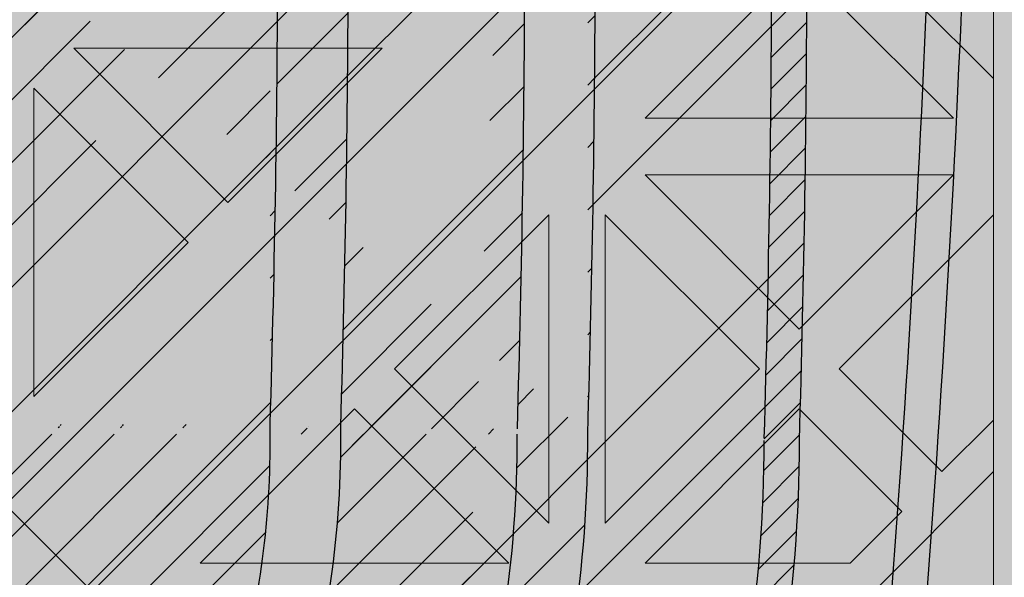
# Model space of a CAD drawing. Units: inches. Extents: x 844 to 2234, y 346 to 1084.
# Tile 54 of 93: x 1869.404 to 1873.853, y 696.327 to 698.846. Entities that reach past the tile are written whole.
import ezdxf

# ---------------------------------------------------------------- set-up
doc = ezdxf.new("R2010")
doc.units = ezdxf.units.IN
doc.header["$MEASUREMENT"] = 0
doc.layers.add('furniture', color=8, linetype='Continuous', lineweight=18)
doc.layers.add('RA-AP-01$0$INT', color=35, linetype='Continuous', lineweight=5)
doc.layers.add('RA-AP-01$0$FURN', color=3, linetype='Continuous')
doc.layers.add('RA-AP-01$0$WOOD', color=64, linetype='Continuous')

# ---------------------------------------------------------------- blocks, each defined once
blk = doc.blocks.new('A$C18D01794')
at = {"layer": 'RA-AP-01$0$INT'}
blk.add_hatch(color=256, dxfattribs=at).paths.add_polyline_path([(4.505206456958071, -6.306712009588038), (5.305206456958072, -6.306712009588038), (5.305206456958072, -7.106712009588038), (5.255206456951893, -7.10671200958804), (5.25520645694868, -6.356712009605972), (4.555206456959269, -6.356712009587461), (4.555206456956052, -7.106712009588038), (4.505206456958073, -7.106712009588038)])
h = blk.add_hatch(color=256, dxfattribs=at)
h.paths.add_polyline_path([(4.585917135068449, -6.356712009588271), (4.555206456959269, -6.35671200958746), (4.555206456959137, -6.387422687716308), (4.874495778835233, -6.706712009592356), (4.90520645695423, -6.676001331474049)])
h.paths.add_polyline_path([(5.255206456948813, -6.387422687716306), (5.255206456948682, -6.356712009605972), (5.224495778822613, -6.356712009605161), (4.905206456953498, -6.676001331474273), (4.935917135072151, -6.706712009592924)])
h.paths.add_polyline_path([(4.935917135072559, -6.706712009592068), (4.905206456953564, -6.737422687710376), (5.255206456951813, -7.087422687708613), (5.255206456951549, -7.026001331471008)])
h.paths.add_polyline_path([(4.555206456956399, -7.026001331471013), (4.555206456956134, -7.087422687708616), (4.905206456953821, -6.737422687710943), (4.874495778835166, -6.70671200959229)])
h = blk.add_hatch(color=256, dxfattribs=at)
h.paths.add_polyline_path([(4.585917135068448, -6.356712009588273), (4.614201406330596, -6.356712009589021), (4.668846067270487, -6.411356670531338), (4.723490728212344, -6.356712009591912), (4.771774999457151, -6.35671200959319), (4.826419660396886, -6.411356670535356), (4.862780050090322, -6.374996280843536), (4.844495778842715, -6.356712009595112), (4.862780050090411, -6.356712009595595), (4.905206456960182, -6.399138416468211), (4.947632863832445, -6.356712009597838), (4.965917135079675, -6.356712009598322), (4.947632863831759, -6.374996280845421), (4.983993253523576, -6.411356670538857), (5.038637914464627, -6.356712009600247), (5.08692218571208, -6.356712009601523), (5.141566846649976, -6.411356670541852), (5.196211507589851, -6.356712009604411), (5.224495778822615, -6.356712009605161), (4.905206456953975, -6.676001331473793)])
h.paths.add_polyline_path([(4.895206456956031, -6.637717060225675), (4.895206456958921, -6.528427738347902), (4.840561796018589, -6.583072399285802)], flags=16)
h.paths.add_polyline_path([(4.915206456955638, -6.637717060226121), (4.969851117895509, -6.583072399288678), (4.915206456957609, -6.528427738348344)], flags=16)
h.paths.add_polyline_path([(4.826419660395175, -6.568930263661755), (4.881064321335613, -6.514285602723745), (4.771774999456703, -6.514285602720857)], flags=16)
h.paths.add_polyline_path([(4.983993253519558, -6.568930263665262), (5.038637914460456, -6.514285602726792), (4.929348592581548, -6.514285602724816)], flags=16)
h.paths.add_polyline_path([(4.881064321336025, -6.494285602723742), (4.826419660397532, -6.439640941782821), (4.771774999457062, -6.494285602720859)], flags=16)
h.paths.add_polyline_path([(4.929348592582019, -6.494285602724817), (5.038637914460982, -6.494285602726792), (4.983993253522945, -6.439640941786327)], flags=16)
h.paths.add_polyline_path([(4.895206456960191, -6.480143467100443), (4.895206456962115, -6.407422687715913), (4.876922185715016, -6.389138416467584), (4.840561796021581, -6.425498806159401)], flags=16)
h.paths.add_polyline_path([(4.915206456958487, -6.480143467100889), (4.969851117899527, -6.425498806162279), (4.933490728206909, -6.389138416468043), (4.9152064569598, -6.40742268771434)], flags=16)
h.paths.add_polyline_path([(4.757632863832376, -6.480143467096812), (4.812277524772842, -6.425498806158772), (4.757632863834348, -6.370854145217844)], flags=16)
h.paths.add_polyline_path([(4.737632863832376, -6.480143467096286), (4.737632863834348, -6.370854145217375), (4.682988202893906, -6.425498806155385)], flags=16)
h.paths.add_polyline_path([(5.05278005008503, -6.480143467103376), (5.052780050087917, -6.370854145224413), (4.998135389146995, -6.425498806162908)], flags=16)
h.paths.add_polyline_path([(5.072780050085024, -6.480143467103744), (5.127424711025931, -6.42549880616527), (5.072780050087916, -6.370854145224832)], flags=16)
h.paths.add_polyline_path([(4.935917135072783, -6.706712009592292), (5.255206456948811, -6.387422687716309), (5.255206456948932, -6.415706958964177), (5.200561796010279, -6.470351619902839), (5.255206456949403, -6.524996280841948), (5.25520645694961, -6.5732805520894), (5.200561796009787, -6.627925213029239), (5.236922185702417, -6.664285602721864), (5.255206456949919, -6.646001331474357), (5.255206456949998, -6.664285602721898), (5.212780050078687, -6.706712009592262), (5.25520645695036, -6.749138416463932), (5.255206456950438, -6.767422687711313), (5.236922185702424, -6.749138416463297), (5.200561796009796, -6.785498806155928), (5.255206456950753, -6.840143467096874), (5.25520645695096, -6.888427738341682), (5.200561796010322, -6.943072399282328), (5.255206456951428, -6.997717060223427), (5.255206456951547, -7.026001331471006)])
h.paths.add_polyline_path([(5.042988202883395, -6.785498806155427), (5.097632863823085, -6.840143467095101), (5.097632863822622, -6.730854145216193)], flags=16)
h.paths.add_polyline_path([(5.028846067259663, -6.771356670531693), (5.083490728198774, -6.716712009592573), (4.974201406321001, -6.716712009593042)], flags=16)
h.paths.add_polyline_path([(5.117632863823087, -6.840143467095186), (5.172277524762331, -6.785498806155926), (5.11763286382262, -6.730854145216225)], flags=16)
h.paths.add_polyline_path([(5.08349072819877, -6.696712009593886), (5.028846067259652, -6.642067348654775), (4.974201406320998, -6.696712009593438)], flags=16)
h.paths.add_polyline_path([(5.131774999446817, -6.854285602718917), (5.186419660386065, -6.799640941779662), (5.241064321325782, -6.854285602719365)], flags=17)
h.paths.add_polyline_path([(5.131774999446228, -6.716712009592374), (5.186419660386065, -6.771356670532194), (5.222780050079488, -6.734996280838764), (5.204495778832781, -6.716712009592063)], flags=16)
h.paths.add_polyline_path([(5.097632863822613, -6.682569873970264), (5.097632863823061, -6.573280552091354), (5.042988202883383, -6.627925213031044)], flags=16)
h.paths.add_polyline_path([(5.131774999446899, -6.874285602718915), (5.241064321325809, -6.874285602719364), (5.186419660386591, -6.928930263658598)], flags=17)
h.paths.add_polyline_path([(5.131774999446226, -6.696712009594078), (5.204495778830767, -6.696712009594374), (5.22278005007868, -6.67842773834687), (5.186419660386049, -6.642067348654249)], flags=16)
h.paths.add_polyline_path([(5.11763286382262, -6.682569873970225), (5.17227752476232, -6.627925213030515), (5.117632863823064, -6.573280552091267)], flags=16)
h.paths.add_polyline_path([(5.186419660386069, -6.613783077405491), (5.241064321325754, -6.559138416465795), (5.131774999446791, -6.559138416466263)], flags=16)
h.paths.add_polyline_path([(5.131774999446872, -6.539138416466263), (5.24106432132578, -6.539138416465794), (5.186419660386554, -6.484493755526573)], flags=16)
h.paths.add_polyline_path([(5.255206456951811, -7.08742268770861), (5.255206456951895, -7.106712009588038), (4.555206456956052, -7.106712009588038), (4.555206456956136, -7.087422687708617), (4.905206456953973, -6.737422687710788)])
h.paths.add_polyline_path([(4.983993253513404, -6.8444937555241), (4.92934859257295, -6.899138416462108), (5.03863791445186, -6.899138416465014)], flags=16)
h.paths.add_polyline_path([(4.969851117889988, -6.83035161990006), (4.915206456952556, -6.775706958960171), (4.915206456949648, -6.884996280837944)], flags=16)
h.paths.add_polyline_path([(4.929348592572535, -6.919138416462105), (4.983993253511019, -6.973783077403037), (5.038637914451496, -6.919138416465012)], flags=16)
h.paths.add_polyline_path([(5.052780050074912, -6.93328055208906), (4.998135389134438, -6.987925213027088), (5.052780050072919, -7.042569873968025)], flags=16)
h.paths.add_polyline_path([(5.07278005007491, -6.933280552089588), (5.072780050072918, -7.042569873968497), (5.127424711013374, -6.987925213030498)], flags=16)
h.paths.add_polyline_path([(4.89520645695295, -6.775706958959721), (4.840561796013067, -6.830351619897157), (4.895206456950961, -6.884996280837494)], flags=16)
h.paths.add_polyline_path([(4.915206456948365, -6.933280552085403), (4.915206456946434, -7.006001331471951), (4.933490728192729, -7.024285602719066), (4.969851117886972, -6.987925213026453)], flags=16)
h.paths.add_polyline_path([(4.881064321327021, -6.899138416461022), (4.82641966038902, -6.84449375552057), (4.771774999448108, -6.899138416459029)], flags=16)
h.paths.add_polyline_path([(4.895206456950073, -6.933280552084951), (4.840561796009022, -6.987925213023558), (4.876922185700835, -7.024285602716997), (4.895206456948749, -7.006001331469487)], flags=16)
h.paths.add_polyline_path([(4.983993253510392, -7.0020673486505), (4.947632863816944, -7.038427738342319), (4.965917135064043, -7.05671200959023), (5.038637914448995, -7.056712009591555)], flags=16)
h.paths.add_polyline_path([(4.881064321326543, -6.91913841646102), (4.771774999447578, -6.919138416459031), (4.826419660385607, -6.973783077399508)], flags=16)
h.paths.add_polyline_path([(4.905206456946447, -7.014285602717636), (4.862780050074785, -7.056712009588352), (4.947632863816685, -7.056712009589775)], flags=16)
h.paths.add_polyline_path([(5.14156684663679, -7.002067348654549), (5.086922185696452, -7.056712009592438), (5.196211507574223, -7.056712009594425)], flags=16)
h.paths.add_polyline_path([(4.8264196603837, -7.002067348646972), (4.771774999442643, -7.056712009585575), (4.8444957788276, -7.056712009587508), (4.862780050075511, -7.038427738340416)], flags=16)
h.paths.add_polyline_path([(4.812277524760289, -6.98792521302292), (4.757632863822258, -6.933280552082447), (4.757632863819352, -7.042569873961408)], flags=16)
h.paths.add_polyline_path([(4.73763286382226, -6.933280552082079), (4.682988202881349, -6.987925213020536), (4.737632863819352, -7.04256987396099)], flags=16)
h.paths.add_polyline_path([(4.723490728195188, -7.056712009584289), (4.668846067257299, -7.002067348643949), (4.614201406317417, -7.056712009581383)], flags=16)
h.paths.add_polyline_path([(4.597632863829262, -6.706712009592262), (4.555206456957951, -6.664285602721896), (4.555206456958029, -6.646001331474357), (4.573490728205535, -6.664285602721864), (4.609851117898167, -6.627925213029238), (4.555206456958338, -6.573280552089402), (4.555206456958546, -6.524996280841952), (4.60985111789767, -6.470351619902839), (4.555206456959015, -6.415706958964177), (4.555206456959138, -6.387422687716309), (4.874495778835167, -6.70671200959229), (4.5552064569564, -7.026001331471015), (4.555206456956523, -6.997717060223433), (4.609851117897629, -6.94307239928233), (4.555206456956988, -6.888427738341681), (4.555206456957198, -6.840143467096881), (4.609851117898153, -6.78549880615593), (4.573490728205528, -6.749138416463297), (4.555206456957507, -6.76742268771132), (4.555206456957585, -6.749138416463933)])
h.paths.add_polyline_path([(4.712780050085332, -6.730854145216195), (4.712780050084863, -6.840143467095105), (4.767424711024555, -6.785498806155427)], flags=16)
h.paths.add_polyline_path([(4.726922185709173, -6.716712009592573), (4.781566846648288, -6.771356670531693), (4.836211507586949, -6.716712009593043)], flags=16)
h.paths.add_polyline_path([(4.692780050085327, -6.730854145216225), (4.638135389145619, -6.785498806155928), (4.692780050084865, -6.840143467095185)], flags=16)
h.paths.add_polyline_path([(4.726922185709182, -6.696712009593886), (4.836211507586949, -6.696712009593436), (4.7815668466483, -6.642067348654773)], flags=16)
h.paths.add_polyline_path([(4.678637914461726, -6.71671200959237), (4.605917135075169, -6.716712009592063), (4.587632863828464, -6.734996280838766), (4.623993253521887, -6.771356670532195)], flags=16)
h.paths.add_polyline_path([(4.712780050085336, -6.68256987397026), (4.767424711024568, -6.627925213031042), (4.71278005008489, -6.573280552091352)], flags=16)
h.paths.add_polyline_path([(4.678637914461726, -6.696712009594076), (4.623993253521899, -6.642067348654247), (4.587632863829271, -6.67842773834687), (4.605917135077185, -6.696712009594376)], flags=16)
h.paths.add_polyline_path([(4.692780050085336, -6.682569873970228), (4.692780050084889, -6.573280552091267), (4.638135389145632, -6.627925213030515)], flags=16)
h.paths.add_polyline_path([(4.623993253521885, -6.799640941779662), (4.678637914461131, -6.854285602718915), (4.56934859258217, -6.854285602719365)], flags=17)
h.paths.add_polyline_path([(4.623993253521901, -6.613783077405509), (4.678637914461158, -6.559138416466263), (4.569348592582195, -6.559138416465795)], flags=16)
h.paths.add_polyline_path([(4.678637914461051, -6.874285602718915), (4.623993253521361, -6.928930263658598), (4.569348592582143, -6.874285602719364)], flags=17)
h.paths.add_polyline_path([(4.678637914461076, -6.539138416466263), (4.623993253521399, -6.484493755526573), (4.569348592582167, -6.539138416465796)], flags=16)
h = blk.add_hatch(color=256, dxfattribs=at)
h.paths.add_polyline_path([(5.028846067259997, -6.642067348655121), (4.974201406321342, -6.696712009593783), (5.083490728199115, -6.69671200959423)])
h.paths.add_polyline_path([(4.974201406321344, -6.716712009593388), (5.028846067260004, -6.771356670532039), (5.083490728199117, -6.716712009592919)])
h.paths.add_polyline_path([(5.042988202883738, -6.785498806155768), (5.097632863823428, -6.840143467095449), (5.097632863822963, -6.73085414521654)])
h.paths.add_polyline_path([(5.117632863822961, -6.730854145216568), (5.117632863823428, -6.840143467095531), (5.172277524762674, -6.785498806156272)])
h.paths.add_polyline_path([(5.131774999446572, -6.716712009592718), (5.186419660386406, -6.77135667053254), (5.222780050079831, -6.734996280839116), (5.204495778833122, -6.716712009592409)])
h.paths.add_polyline_path([(5.236922185702764, -6.749138416463644), (5.200561796010139, -6.785498806156274), (5.255206456949971, -6.840143467096101), (5.255206456950271, -6.76742268771115)])
h.paths.add_polyline_path([(5.186419660386412, -6.799640941780006), (5.131774999447164, -6.854285602719262), (5.241064321326123, -6.854285602719711)])
h.paths.add_polyline_path([(5.131774999447238, -6.874285602719261), (5.186419660386934, -6.928930263658944), (5.241064321326153, -6.874285602719709)])
h.paths.add_polyline_path([(5.200561796010663, -6.943072399282675), (5.255206456949324, -6.997717060221329), (5.255206456949777, -6.888427738343558)])
h.paths.add_polyline_path([(5.21278005007903, -6.706712009592607), (5.255206456950223, -6.749138416463798), (5.255206456950696, -6.664285602721891)])
h.paths.add_polyline_path([(5.13177499944657, -6.696712009594424), (5.204495778831106, -6.696712009594723), (5.222780050079024, -6.678427738347219), (5.186419660386397, -6.642067348654592)])
h.paths.add_polyline_path([(5.117632863823405, -6.573280552091611), (5.117632863822955, -6.682569873970578), (5.172277524762665, -6.627925213030859)])
h.paths.add_polyline_path([(5.042988202883727, -6.627925213031387), (5.097632863822957, -6.682569873970603), (5.097632863823407, -6.573280552091697)])
h.paths.add_polyline_path([(5.131774999447135, -6.559138416466609), (5.186419660386394, -6.613783077405857), (5.241064321326097, -6.559138416466144)])
h.paths.add_polyline_path([(5.200561796010128, -6.627925213029584), (5.236922185702758, -6.664285602722211), (5.255206456950264, -6.646001331474705), (5.255206456949948, -6.573280552089752)])
h.paths.add_polyline_path([(5.186419660386895, -6.484493755526919), (5.131774999447213, -6.539138416466609), (5.241064321326127, -6.539138416466142)])
h.paths.add_polyline_path([(5.200561796010624, -6.470351619903183), (5.255206456949745, -6.524996280842298), (5.255206456949276, -6.415706958964523)])
h = blk.add_hatch(color=256, dxfattribs=at)
h.paths.add_polyline_path([(4.905206456953579, -6.70671200959253), (4.905206456953751, -6.676001331474523), (4.874495778835229, -6.706712009592358)])
h.paths.add_polyline_path([(4.935917135071924, -6.706712009592703), (4.905206456953583, -6.706712009592529), (4.90520645695341, -6.737422687710532)])
h = blk.add_hatch(color=256, dxfattribs=at)
h.paths.add_polyline_path([(4.895206456952951, -6.77570695895972), (4.840561796013068, -6.830351619897156), (4.895206456950958, -6.884996280837495)])
h.paths.add_polyline_path([(4.915206456949649, -6.884996280837942), (4.969851117889987, -6.830351619900054), (4.915206456952556, -6.775706958960171)])
h.paths.add_polyline_path([(5.038637914451862, -6.899138416465013), (4.983993253513403, -6.8444937555241), (4.929348592572953, -6.899138416462106)])
h.paths.add_polyline_path([(4.929348592572535, -6.919138416462105), (4.983993253511018, -6.973783077403037), (5.038637914451497, -6.919138416465012)])
h.paths.add_polyline_path([(4.915206456948366, -6.933280552085397), (4.915206456946433, -7.006001331471951), (4.93349072819273, -7.024285602719068), (4.969851117886972, -6.987925213026454)])
h.paths.add_polyline_path([(5.038637914448995, -7.056712009591553), (4.983993253510389, -7.002067348650502), (4.947632863816946, -7.038427738342318), (4.965917135064043, -7.05671200959023)])
h.paths.add_polyline_path([(5.05278005007292, -7.042569873968023), (5.05278005007491, -6.933280552089059), (4.998135389134438, -6.987925213027088)])
h.paths.add_polyline_path([(5.07278005007292, -7.042569873968496), (5.127424711013374, -6.987925213030498), (5.072780050074909, -6.933280552089588)])
h.paths.add_polyline_path([(5.141566846636789, -7.002067348654547), (5.086922185696449, -7.056712009592438), (5.196211507574223, -7.056712009594425)])
h.paths.add_polyline_path([(4.947632863816688, -7.056712009589774), (4.905206456946449, -7.014285602717634), (4.862780050074784, -7.056712009588353)])
h.paths.add_polyline_path([(4.840561796009025, -6.987925213023556), (4.876922185700834, -7.024285602716997), (4.895206456948747, -7.006001331469488), (4.895206456950075, -6.933280552084953)])
h.paths.add_polyline_path([(4.88106432132654, -6.919138416461021), (4.771774999447577, -6.919138416459031), (4.826419660385606, -6.973783077399508)])
h.paths.add_polyline_path([(4.881064321327019, -6.899138416461022), (4.826419660389019, -6.844493755520571), (4.771774999448108, -6.89913841645903)])
h.paths.add_polyline_path([(4.757632863819352, -7.042569873961409), (4.812277524760284, -6.987925213022922), (4.757632863822259, -6.933280552082447)])
h.paths.add_polyline_path([(4.8264196603837, -7.002067348646974), (4.771774999442646, -7.056712009585575), (4.844495778827599, -7.05671200958751), (4.862780050075512, -7.038427738340417)])
h.paths.add_polyline_path([(4.737632863819352, -7.042569873960988), (4.737632863822258, -6.933280552082078), (4.682988202881349, -6.987925213020538)])
h.paths.add_polyline_path([(4.668846067257299, -7.002067348643952), (4.61420140631742, -7.056712009581384), (4.723490728195189, -7.056712009584292)])
for p, q in [((5.255206456951895, -7.106712009588038), (5.255206456948681, -6.356712009605972)), ((5.25520645694988, -6.74913841646345), (5.255206456950353, -6.664285602721543)), ((4.935917135071927, -6.706712009592701), (4.905206456953407, -6.737422687710532)), ((4.935917135072783, -6.706712009592292), (5.255206456951548, -7.026001331471007)), ((5.212780050078687, -6.706712009592262), (5.25520645694988, -6.74913841646345)), ((5.083490728198772, -6.716712009592574), (4.974201406321001, -6.716712009593042)), ((4.974201406321001, -6.716712009593042), (5.028846067259663, -6.771356670531693)), ((5.08349072819877, -6.716712009592578), (5.028846067259663, -6.771356670531693)), ((5.131774999446229, -6.716712009592372), (5.186419660386063, -6.771356670532195)), ((5.204495778831181, -6.716712009592063), (5.131774999446229, -6.716712009592372)), ((5.204495778832774, -6.716712009592056), (5.222780050080282, -6.73499628083956)), ((5.09763286382262, -6.730854145216195), (5.042988202883395, -6.785498806155425)), ((5.097632863823085, -6.840143467095105), (5.09763286382262, -6.730854145216195)), ((5.11763286382262, -6.730854145216223), (5.172277524762331, -6.785498806155928)), ((5.117632863823085, -6.840143467095186), (5.11763286382262, -6.730854145216223)), ((5.186419660386062, -6.771356670532195), (5.222780050078687, -6.734996280839565)), ((4.905206456953975, -6.737422687710788), (5.255206456951811, -7.087422687708611)), ((5.200561796009796, -6.78549880615593), (5.236922185702423, -6.749138416463297)), ((5.255206456949928, -6.767422687710803), (5.236922185702423, -6.749138416463296)), ((5.236922185702423, -6.749138416463297), (5.25520645694988, -6.767422687710757)), ((5.255206456949927, -6.767422687710803), (5.255206456949628, -6.840143467095755)), ((4.915206456952556, -6.775706958960171), (4.969851117889986, -6.830351619900053)), ((4.915206456949648, -6.884996280837942), (4.915206456952556, -6.775706958960171)), ((5.042988202883397, -6.785498806155427), (5.097632863823085, -6.840143467095105)), ((5.117632863823085, -6.840143467095186), (5.172277524762331, -6.785498806155928)), ((5.255206456949628, -6.840143467095755), (5.200561796009796, -6.785498806155928)), ((5.131774999446817, -6.854285602718915), (5.186419660386065, -6.799640941779662)), ((5.24106432132578, -6.854285602719365), (5.186419660386065, -6.799640941779662)), ((4.915206456949651, -6.88499628083794), (4.969851117889986, -6.830351619900053)), ((4.929348592572952, -6.899138416462106), (4.983993253513403, -6.844493755524101)), ((4.983993253513404, -6.844493755524103), (5.038637914451862, -6.899138416465012)), ((5.131774999446817, -6.854285602718915), (5.24106432132578, -6.854285602719365)), ((5.131774999446899, -6.874285602718915), (5.241064321325809, -6.874285602719364)), ((5.186419660386587, -6.928930263658596), (5.131774999446899, -6.874285602718915)), ((5.241064321325809, -6.874285602719364), (5.186419660386589, -6.928930263658598)), ((5.255206456949429, -6.888427738343214), (5.200561796010322, -6.943072399282328)), ((5.255206456949433, -6.888427738343212), (5.255206456948982, -6.997717060220983)), ((5.038637914451862, -6.899138416465012), (4.929348592572952, -6.899138416462106))]:
    blk.add_line(p, q, dxfattribs=at)
blk = doc.blocks.new('A$C32926AE1')
at = {"layer": 'RA-AP-01$0$FURN'}
h = blk.add_hatch(dxfattribs=at)
h.set_pattern_fill('ANSI31', color=256, scale=0.1, style=0)
h.set_pattern_definition([(45, (0, 0), (-0.0088388347648318, 0.0088388347648318), [])])
edge = h.paths.add_edge_path(flags=16)
edge.add_arc((4.904771284329206, 4.246793130718756), 0.2603971832811541, 75.22398030683196, 104.7760196931204)
edge.add_arc((4.904771284329206, 4.246793130718756), 0.2603971832811541, 75.223980306832, 104.77601969312039, ccw=False)
edge = h.paths.add_edge_path(flags=16)
edge.add_arc((4.904771284329206, 4.067062675376612), 0.2603971832811541, 255.2239803068796, 284.776019693168)
edge.add_arc((4.904771284329206, 4.067062675376612), 0.2603971832811541, 255.22398030687958, 284.77601969316805, ccw=False)
edge = h.paths.add_edge_path(flags=0)
edge.add_arc((4.904771284329206, 4.067062675376612), 0.2603971832811541, 255.2239803068796, 284.776019693168)
edge.add_arc((4.904771284329206, 4.067062675376612), 0.2603971832811541, 255.22398030687958, 284.77601969316805, ccw=False)
edge = h.paths.add_edge_path(flags=0)
edge.add_arc((4.904771284329206, 4.067062675376612), 0.2603971832811541, 255.2239803068796, 284.776019693168)
edge.add_arc((4.904771284329206, 4.067062675376612), 0.2603971832811541, 255.22398030687958, 284.77601969316805, ccw=False)
edge = h.paths.add_edge_path()
edge.add_arc((4.604388392048174, 4.588829985554312), 0.1599999999999918, 342.3781640246255, 354.4317409793762)
edge.add_arc((5.090145208887507, 4.43216705527679), 0.3503971832811637, 162.0091218307731, 180.3186872093483)
edge.add_arc((5.205154176610243, 4.588829985554953), 0.1599999999999917, 185.5682590208461, 197.6218359767349)
edge.add_arc((4.904771284329229, 4.246793130718735), 0.3503971832811761, 72.00912183053516, 107.9908781690354)
edge.add_arc((9.535952835716557, 4.28682295566602), 4.798342501046485, 178.2875002453811, 181.5576802719453)
edge.add_arc((4.719397359771122, 4.43216705527679), 0.3503971832811637, 359.6813127906516, 377.9908781692269)
edge.add_arc((9.535967292294904, 4.286822350292874), 4.778371420254705, 178.2965938931842, 181.5667745797229)
edge.add_arc((4.719397359771122, 4.43216705527679), 0.3303971832811637, 359.6813127906516, 377.9908781692269)
edge.add_arc((0.2735752763637294, 4.286822350292874), 4.7783714202547, 358.4332254202771, 361.7034061068158)
edge.add_arc((5.061434214606998, 4.732549947558029), 0.1600000000000254, 252.3781640250584, 264.4317409792362)
edge.add_arc((4.748108354051257, 4.732549947558012), 0.1600000000000541, 275.5682590208426, 287.6218359759532)
edge.add_arc((4.604388392048115, 4.588829985554317), 0.1800000000000505, 342.3567572500182, 349.3735009646207)
edge.add_arc((5.205154176610254, 4.588829985554976), 0.1800000000000069, 190.6264990356027, 197.6432427513933)
edge.add_arc((5.061434214607106, 4.732549947558013), 0.1800000000000424, 252.3567572496606, 259.3735009644582)
edge.add_arc((4.904771284329208, 4.246793130718737), 0.3303971832811676, 71.99844483668534, 108.0015551637021)
edge.add_arc((4.748108354051414, 4.732549947558045), 0.1800000000000547, 280.6264990355479, 287.6432427495938)
edge.add_arc((5.090145208887514, 4.432167055276789), 0.2803971832811691, 162.8706300666893, 180.816523289902)
edge.add_arc((4.719397359771136, 4.432167055276689), 0.2803971832811534, 359.183476710103, 377.1293699333214)
edge.add_arc((4.904771284329222, 4.246793130718737), 0.2803971832811769, 72.87063006672916, 107.1293699332334)
edge.add_arc((5.090145208887522, 4.432167055276788), 0.2603971832811776, 165.2239803068007, 180.9953123810312)
edge.add_arc((4.719397359771141, 4.432167055276699), 0.2603971832811458, 359.0046876189768, 374.7760196932087)
edge.add_arc((5.090145208887507, 4.43216705527679), 0.3303971832811637, 162.0091218307731, 180.3186872093483)
edge.add_arc((9.53595427642584, 4.285015535491528), 4.728345371032053, 178.265043920078, 181.5679956281801)
edge.add_arc((0.2735882922327999, 4.285015535491582), 4.728345371032045, 358.4320043718193, 361.7349560799204)
edge.add_arc((9.535953591267507, 4.284458026472751), 4.708343996644348, 178.2573054306777, 181.5704995759608)
edge.add_arc((0.273588977391114, 4.284458026472785), 4.708343996644358, 358.4295004240388, 361.7426945693213)
edge.add_arc((0.2735889773911131, 4.029397779622582), 4.708343996644359, 358.2573054306787, 361.5704995759613)
edge.add_arc((9.535953591267518, 4.029397779622618), 4.708343996644359, 178.4295004240391, 181.7426945693223)
edge.add_arc((0.2735882922327901, 4.028840270603786), 4.728345371032054, 358.2650439200796, 361.5679956281808)
edge.add_arc((9.53595427642584, 4.028840270603841), 4.728345371032054, 178.4320043718199, 181.7349560799219)
edge.add_arc((0.2735752763637302, 4.027033455802493), 4.778371420254699, 358.2965938931842, 361.5667745797229)
edge.add_arc((4.719397359771122, 3.881688750818578), 0.3303971832811637, 342.0091218307731, 360.3186872093484)
edge.add_arc((5.090145208887507, 3.881688750818578), 0.3303971832811637, 179.6813127906516, 197.9908781692269)
edge.add_arc((9.535967292294904, 4.027033455802493), 4.778371420254705, 178.433225420277, 181.7034061068158)
edge.add_arc((4.719397359771122, 3.881688750818578), 0.3503971832811637, 342.0091218307731, 360.3186872093484)
edge.add_arc((9.53595283571655, 4.027032850429349), 4.79834250104648, 178.4423197280546, 181.7124997546188)
edge.add_arc((4.719397359771141, 3.881688750818669), 0.2603971832811458, 345.2239803067913, 360.9953123810232)
edge.add_arc((5.090145208887522, 3.88168875081858), 0.2603971832811776, 179.0046876189687, 194.7760196931993)
edge.add_arc((4.904771284329222, 4.067062675376631), 0.2803971832811769, 252.8706300667665, 287.1293699332708)
edge.add_arc((4.719397359771136, 3.881688750818678), 0.2803971832811534, 342.8706300666787, 360.8165232898969)
edge.add_arc((5.090145208887514, 3.881688750818579), 0.2803971832811691, 179.183476710098, 197.1293699333106)
edge.add_arc((4.748108354051414, 3.581305858537323), 0.1800000000000547, 72.3567572504062, 79.37350096445199)
edge.add_arc((4.904771284329208, 4.067062675376631), 0.3303971832811676, 251.9984448362979, 288.0015551633146)
edge.add_arc((5.061434214607106, 3.581305858537355), 0.1800000000000424, 100.6264990355418, 107.6432427503394)
edge.add_arc((5.205154176610254, 3.725025820540392), 0.1800000000000069, 162.3567572486066, 169.3735009643972)
edge.add_arc((4.604388392048115, 3.725025820541051), 0.1800000000000505, 10.62649903537925, 17.64324274998182)
edge.add_arc((4.748108354051257, 3.581305858537356), 0.1600000000000541, 72.37816402404681, 84.43174097915735)
edge.add_arc((4.904771284329229, 4.067062675376632), 0.3503971832811761, 252.0091218309645, 287.9908781694648)
edge.add_arc((5.061434214606998, 3.581305858537339), 0.1600000000000254, 95.56825902076373, 107.6218359749416)
edge.add_arc((5.205154176610243, 3.725025820540414), 0.1599999999999917, 162.3781640232651, 174.4317409791539)
edge.add_arc((5.090145208887507, 3.881688750818578), 0.3503971832811637, 179.6813127906516, 197.9908781692269)
edge.add_arc((4.604388392048174, 3.725025820541056), 0.1599999999999918, 5.568259020623824, 17.62183597537444)
edge.add_arc((0.2735897329420762, 4.28682295566602), 4.798342501046482, 358.4423197280547, 361.7124997546188)
edge.add_arc((0.2735897329420691, 4.027032850429348), 4.798342501046489, 358.2875002453812, 361.5576802719453)
at = {"layer": 'RA-AP-01$0$WOOD'}
h = blk.add_hatch(color=256, dxfattribs=at)
h.dxf.hatch_style = 1
h.paths.add_polyline_path([(5.157430609644524, 4.573483066760929, -0.1009492694046607), (5.155401577623758, 4.593365984175333, -0.1842662638101597), (5.172249623284174, 4.638795604568598, 0.2056608120311276), (5.179560981299304, 4.661316324430096, 0.3614336704623542), (5.134352340494423, 4.706524965234944, 0.2056608120311297), (5.111831620632933, 4.699213607219793, -0.1842662638101113), (5.066402000239693, 4.682365561559342, -0.1055311479399994), (5.045656153913092, 4.68467289944697, 0.1567636581983829), (4.763886414745334, 4.684672899446966, -0.1055311479399895), (4.743140568418733, 4.68236556155934, -0.1842662638100833), (4.6977109480255, 4.69921360721979, 0.2056608120302612), (4.675190228164109, 4.706524965234949, 0.3614336704708441), (4.629981587358889, 4.66131632442871, 0.2056608120245944), (4.637292945374126, 4.638795604567974, -0.1842662638101024), (4.654140991034615, 4.59336598417475, -0.1009492694055169), (4.652111959013835, 4.573483066760181, 0.021410119221476), (4.629748025606143, 4.156712009541676, 0.0214101192214795), (4.652111959013809, 3.739940952323101, -0.1009492694059586), (4.654140991034615, 3.720058034908448, -0.1842662638100975), (4.637292945374126, 3.674628414515226, 0.2056608120245705), (4.629981587358889, 3.652107694654492, 0.3614336704708879), (4.675190228164113, 3.606899053848249, 0.2056608120302384), (4.697710948025501, 3.614210411863408, -0.1842662638100995), (4.743140568418738, 3.63105845752386, -0.1055311479402541), (4.763886414745388, 3.628751119636215, 0.1567636581983776), (5.045656153913137, 3.628751119636244, -0.1055311479397538), (5.066402000239692, 3.631058457523857, -0.1842662638101067), (5.111831620632931, 3.614210411863407, 0.2056608120310924), (5.134352340494417, 3.606899053848256, 0.3614336704624001), (5.179560981299307, 3.652107694653103, 0.2056608120311314), (5.172249623284175, 3.6746284145146, -0.1842662638101402), (5.155401577623758, 3.72005803490786, -0.1009492694051366), (5.15743060964455, 3.739940952322354, 0.0214101192215073), (5.179794543052287, 4.156712009541468, 0.0214101192215252)])
h.paths.add_polyline_path([(4.639748609479751, 4.156712009541513, 0.0213537860821624), (4.661970494867118, 3.741887061152232, -0.094075836301374), (4.664143710413708, 3.7196126951003, -0.1824818158568985), (4.644813765429836, 3.668037719127816, 0.2056608120245319), (4.639939526753007, 3.653023905887301, 0.3614336704710246), (4.676106439397173, 3.616856993242342, 0.2056608120302234), (4.691120252638095, 3.621731231919122, -0.1824818158602558), (4.742695228611606, 3.641061176902986, -0.1029891339458722), (4.766991894714349, 3.638256818950944, 0.156709409989566), (5.042550673941472, 3.638256818950105, -0.102989133958497), (5.066847340047078, 3.641061176902949, -0.1824818158594995), (5.118422316020358, 3.621731231919103, 0.2056608120311416), (5.133436129261316, 3.616856993242346, 0.3614336704621468), (5.169603041905217, 3.653023905886178, 0.2056608120310986), (5.164728803228477, 3.668037719127177, -0.1824818158565612), (5.145398858244737, 3.719612695099578, -0.0940758363009313), (5.147572073791232, 3.741887061151398, 0.0213537860822023), (5.169793959178681, 4.156712009541451, 0.0213537860822226), (5.147572073791203, 4.571536957931898, -0.0940758363005034), (5.145398858244737, 4.59381132398362, -0.1824818158565587), (5.164728803228476, 4.645386299956021, 0.2056608120311045), (5.169603041905216, 4.66040011319702, 0.3614336704621845), (5.133436129261313, 4.696567025840856, 0.2056608120310773), (5.118422316020359, 4.691692787164098, -0.182481815859508), (5.066847340047078, 4.67236284218025, -0.1029891339584606), (5.04255067394148, 4.675167200133092, 0.156709409989566), (4.766991894714357, 4.675167200132257, -0.1029891339458842), (4.742695228611611, 4.672362842180213, -0.1824818158602725), (4.691120252638095, 4.691692787164077, 0.2056608120302152), (4.676106439397174, 4.696567025840858, 0.3614336704710363), (4.639939526753005, 4.660400113195899, 0.2056608120245495), (4.644813765429837, 4.645386299955384, -0.1824818158568934), (4.664143710413708, 4.593811323982902, -0.0940758363009187), (4.661970494867149, 4.571536957931074, 0.021353786082177)], flags=16)
h.paths.add_polyline_path([(5.129794543052235, 4.432167055276933, -0.0141661062790638), (5.130152669293814, 4.156927903047693, -0.0141661062790647), (5.129794543052234, 3.881688750818433, -0.0785247771143638), (5.10979738006795, 3.755143611847103, 0.0945969212073497), (5.105408519571111, 3.717898134952927, 0.1043170707844957), (5.116074640131521, 3.670385395016088, 0.1043170707864965), (5.068561900193738, 3.681051515576561, 0.09459692119553), (5.031316423304057, 3.676662655080835, -0.1580239521427272), (4.778226145355827, 3.676662655080367, 0.0945969211986668), (4.740980668464973, 3.681051515576592, 0.1043170707882822), (4.693467928526415, 3.670385395015844, 0.1043170707867916), (4.704134049087309, 3.717898134953662, 0.0945969211972894), (4.69974518859162, 3.755143611844042, -0.0785247771163196), (4.679748025606343, 3.881688750818406, -0.0141661062790663), (4.679389899364763, 4.156927903047693, -0.0141661062790672), (4.679748025606343, 4.432167055276998, -0.0785247771163064), (4.699745188591625, 4.55871219425134, 0.094596921197333), (4.704134049087308, 4.595957671141738, 0.1043170707867205), (4.693467928526416, 4.643470411079523, 0.1043170707882628), (4.740980668464965, 4.632804290518776, 0.0945969211988114), (4.778226145355874, 4.637193151015016, -0.158023952142669), (5.031316423304015, 4.637193151014546, 0.0945969211956361), (5.068561900193736, 4.632804290518806, 0.1043170707864979), (5.11607464013152, 4.643470411079278, 0.1043170707844617), (5.105408519571112, 4.595957671142455, 0.0945969212074597), (5.109797380067959, 4.558712194248236, -0.0785247771143467)], flags=0)
h.paths.add_polyline_path([(5.119794532311105, 4.432259799204851, -0.0142000800617244), (5.120156169157484, 4.156927903047701, -0.0142000800617277), (5.119794532311105, 3.881596006890482, -0.0784894509520253), (5.100273383573699, 3.758192358677797, 0.0940138827242913), (5.095413455884425, 3.717477693979438, 0.0606271852308753), (5.099615656341024, 3.686844378806616, 0.0606271852322524), (5.068982341167493, 3.691046579263239, 0.0940138827010453), (5.028267676478798, 3.686186651576848, -0.1580706864508061), (4.781274892180912, 3.686186651576435, 0.0940138827026903), (4.740560227491556, 3.691046579263279, 0.0606271852339895), (4.709926912317155, 3.686844378806508, 0.0606271852329405), (4.714129112773991, 3.717477693980356, 0.094013882701304), (4.709269185087677, 3.758192358669163, -0.0784894509577193), (4.689748036347473, 3.881596006890469, -0.014200080061729), (4.689386399501094, 4.156927903047709, -0.0142000800617217), (4.689748036347473, 4.432259799204808, -0.078489450957724), (4.709269185087651, 4.555663447426125, 0.0940138827014585), (4.714129112773992, 4.596378112114996, 0.0606271852329731), (4.709926912317154, 4.62701142728886, 0.0606271852340196), (4.74056022749157, 4.622809226832087, 0.0940138827024997), (4.781274892180847, 4.627669154518912, -0.1580706864508359), (5.028267676478777, 4.627669154518526, 0.0940138827010946), (5.068982341167492, 4.622809226832129, 0.060627185232254), (5.099615656341024, 4.627011427288751, 0.0606271852308727), (5.095413455884425, 4.59637811211593, 0.0940138827241088), (5.100273383573675, 4.555663447417647, -0.0784894509520978)], flags=0)
h.paths.add_polyline_path([(5.06978912287499, 4.430218106756144, -0.014241683694547), (5.070173729147532, 4.156927903047672, -0.0142416836945458), (5.06978912287499, 3.883637699339223, -0.0800609523125196), (5.052662118612511, 3.773463122773442, 0.0526421978001116), (5.04590916754064, 3.740550867606997, 0.0526421977992423), (5.012996912374707, 3.73379791653534, -0.1583028414718258), (4.796545656286308, 3.73379791653451, 0.0526421978034211), (4.763633401117837, 3.740550867607021, 0.0526421978018622), (4.756880450045755, 3.773463122774558, -0.0800609523117106), (4.739753445783639, 3.883637699339268, -0.0142416836945435), (4.739368839511098, 4.156927903047671, -0.0142416836945477), (4.739753445783639, 4.430218106756155, -0.0800609523116345), (4.75688045004574, 4.540392683320762, 0.052642197801941), (4.763633401117837, 4.573304938488346, 0.0526421978035071), (4.796545656286361, 4.580057889560873, -0.1583028414717561), (5.012996912374669, 4.580057889560039, 0.0526421977993048), (5.04590916754064, 4.57330493848837, 0.0526421978002057), (5.052662118612529, 4.540392683321868, -0.080060952312477)], flags=0)
h.paths.add_polyline_path([(5.049789715110557, 4.43038092723357, -0.0143097550741839), (5.05018085590259, 4.156927903047715, -0.0143097550741854), (5.049789715110558, 3.883474878861827, -0.0800685599149176), (5.03362098255317, 3.779581877367999, 0.0306258898956367), (5.028241146483733, 3.758218888663947, 0.0306258898977031), (5.006878157778253, 3.75283905259408, -0.1583983521624096), (4.802664410878162, 3.752839052594731, 0.0306258898946014), (4.781301422174808, 3.758218888663924, 0.0306258898967912), (4.775921586105202, 3.779581877368794, -0.080068559914251), (4.759752853548071, 3.883474878861786, -0.0143097550741854), (4.759361712756037, 4.156927903047671, -0.0143097550741854), (4.759752853548071, 4.430380927233557, -0.0800685599142479), (4.775921586105193, 4.534273928726546, 0.0306258898968306), (4.781301422174808, 4.555636917431444, 0.0306258898945754), (4.802664410878143, 4.561016753500631, -0.1583983521624168), (5.006878157778244, 4.561016753501291, 0.0306258898977177), (5.028241146483733, 4.555636917431421, 0.0306258898958182), (5.03362098255321, 4.534273928727244, -0.080068559914796)], flags=0)
h.paths.add_polyline_path([(4.999766070382627, 4.428171244713864, -0.0143443147609634), (5.000198441819402, 4.156927903047689, -0.0143443147609612), (4.999766070382627, 3.885684561381556, -0.0784641635803329), (4.987356730658798, 3.799103304488872, -0.1506053783831347), (4.822185837999821, 3.79910330448882, -0.0784641635803318), (4.809776498276007, 3.885684561381509, -0.014344314760963), (4.809344126839227, 4.156927903047677, -0.0143443147609645), (4.809776498276007, 4.428171244713873, -0.0784641635803192), (4.822185837999822, 4.514752501606549, -0.1506053783831338), (4.987356730658798, 4.514752501606494, -0.078464163580285)], flags=0)
h.paths.add_polyline_path([(4.979755254238824, 4.42764379880488, -0.0143772539198268), (4.980205517789977, 4.156927903047693, -0.0143772539198275), (4.979755254238824, 3.886212007290489, -0.0689242507424422), (4.971183264704897, 3.815276770442801, -0.1296645318904179), (4.838359303953726, 3.815276770442746, -0.0689242507424186), (4.829787314419809, 3.886212007290419, -0.0143772539198292), (4.829337050868653, 4.156927903047653, -0.0143772539198325), (4.829787314419809, 4.427643798804946, -0.0689242507424211), (4.838359303953725, 4.498579035652621, -0.1296645318904187), (4.971183264704897, 4.498579035652565, -0.0689242507424401)], flags=0)
h = blk.add_hatch(color=256, dxfattribs=at)
h.dxf.hatch_style = 1
h.paths.add_polyline_path([(5.145398858244737, 4.59381132398362, -0.1824818158565616), (5.164728803228476, 4.645386299956021, 0.2056608120311045), (5.169603041905216, 4.66040011319702, 0.3614336704621845), (5.133436129261313, 4.696567025840856, 0.2056608120310773), (5.118422316020359, 4.691692787164098, -0.182481815859508), (5.066847340047078, 4.67236284218025, -0.1029891339584606), (5.04255067394148, 4.675167200133092, 0.156709409989566), (4.766991894714357, 4.675167200132257, -0.1029891339458842), (4.742695228611611, 4.672362842180213, -0.1824818158602725), (4.691120252638095, 4.691692787164077, 0.2056608120302152), (4.676106439397174, 4.696567025840858, 0.3614336704710363), (4.639939526753005, 4.660400113195899, 0.2056608120245495), (4.644813765429837, 4.645386299955384, -0.1824818158568934), (4.664143710413708, 4.593811323982902, -0.0940758363009187), (4.661970494867149, 4.571536957931074, 0.0213537860821772), (4.639748609479751, 4.156712009541507, 0.0213537860821625), (4.661970494867119, 3.741887061152226, -0.0940758363013071), (4.664143710413708, 3.719612695100309, -0.1824818158569294), (4.644813765429836, 3.668037719127816, 0.2056608120245319), (4.639939526753007, 3.653023905887301, 0.3614336704710246), (4.676106439397173, 3.616856993242342, 0.2056608120302234), (4.691120252638095, 3.621731231919122, -0.1824818158602558), (4.742695228611606, 3.641061176902986, -0.1029891339458722), (4.766991894714349, 3.638256818950944, 0.156709409989566), (5.042550673941472, 3.638256818950105, -0.102989133958497), (5.066847340047078, 3.641061176902949, -0.1824818158594995), (5.118422316020358, 3.621731231919103, 0.2056608120311416), (5.133436129261316, 3.616856993242346, 0.3614336704621468), (5.169603041905217, 3.653023905886178, 0.2056608120310986), (5.164728803228477, 3.668037719127177, -0.1824818158565612), (5.145398858244737, 3.719612695099578, -0.0940758363009313), (5.147572073791232, 3.741887061151398, 0.0213537860822023), (5.169793959178681, 4.156712009541451, 0.0213537860822226), (5.147572073791203, 4.571536957931898, -0.0940758363004996)])
h.paths.add_polyline_path([(5.109797380067958, 4.55871219424824, -0.0785247771143472), (5.129794543052234, 4.432167055276936, -0.0141661062790644), (5.130152669293814, 4.156927903047685, -0.014166106279066), (5.129794543052234, 3.881688750818401, -0.0785247771143517), (5.109797380067946, 3.755143611847092, 0.0945969212073132), (5.105408519571111, 3.717898134952929, 0.1043170707844995), (5.116074640131521, 3.670385395016088, 0.1043170707864965), (5.068561900193738, 3.681051515576561, 0.09459692119553), (5.031316423304057, 3.676662655080835, -0.1580239521427272), (4.778226145355827, 3.676662655080367, 0.0945969211986668), (4.740980668464973, 3.681051515576592, 0.1043170707882822), (4.693467928526415, 3.670385395015844, 0.1043170707867916), (4.704134049087309, 3.717898134953662, 0.0945969211972894), (4.69974518859162, 3.755143611844042, -0.0785247771163196), (4.679748025606343, 3.881688750818406, -0.0141661062790663), (4.679389899364763, 4.156927903047693, -0.0141661062790672), (4.679748025606343, 4.432167055276998, -0.0785247771163064), (4.699745188591625, 4.55871219425134, 0.094596921197333), (4.704134049087308, 4.595957671141738, 0.1043170707867205), (4.693467928526416, 4.643470411079523, 0.1043170707882628), (4.740980668464965, 4.632804290518776, 0.0945969211988114), (4.778226145355874, 4.637193151015016, -0.158023952142669), (5.031316423304015, 4.637193151014546, 0.0945969211956361), (5.068561900193736, 4.632804290518806, 0.1043170707864979), (5.11607464013152, 4.643470411079278, 0.1043170707844617), (5.105408519571112, 4.595957671142455, 0.0945969212074504)], flags=16)
h.paths.add_polyline_path([(5.100273383573655, 4.55566344741771, -0.0784894509521388), (5.119794532311105, 4.432259799204852, -0.0142000800617252), (5.120156169157484, 4.156927903047686, -0.014200080061726), (5.119794532311105, 3.881596006890502, -0.0784894509520446), (5.100273383573696, 3.758192358677786, 0.0940138827242721), (5.095413455884425, 3.717477693979436, 0.0606271852308692), (5.099615656341024, 3.686844378806616, 0.0606271852322522), (5.068982341167493, 3.691046579263239, 0.0940138827010453), (5.028267676478798, 3.686186651576848, -0.1580706864508061), (4.781274892180912, 3.686186651576435, 0.0940138827026903), (4.740560227491556, 3.691046579263279, 0.0606271852339895), (4.709926912317155, 3.686844378806508, 0.0606271852329405), (4.714129112773991, 3.717477693980356, 0.094013882701304), (4.709269185087677, 3.758192358669163, -0.0784894509577193), (4.689748036347473, 3.881596006890469, -0.014200080061729), (4.689386399501094, 4.156927903047709, -0.0142000800617217), (4.689748036347473, 4.432259799204808, -0.078489450957724), (4.709269185087651, 4.555663447426125, 0.0940138827014585), (4.714129112773992, 4.596378112114996, 0.0606271852329731), (4.709926912317154, 4.62701142728886, 0.0606271852340196), (4.74056022749157, 4.622809226832087, 0.0940138827024997), (4.781274892180847, 4.627669154518912, -0.1580706864508359), (5.028267676478777, 4.627669154518526, 0.0940138827010946), (5.068982341167492, 4.622809226832129, 0.060627185232254), (5.099615656341024, 4.627011427288751, 0.0606271852308727), (5.095413455884425, 4.59637811211593, 0.094013882723957)], flags=0)
h.paths.add_polyline_path([(5.04590916754064, 4.57330493848837, 0.0526421978002057), (5.052662118612529, 4.540392683321868, -0.0800609523124783), (5.06978912287499, 4.430218106756142, -0.0142416836945469), (5.070173729147532, 4.156927903047672, -0.0142416836945458), (5.06978912287499, 3.883637699339223, -0.0800609523125196), (5.052662118612511, 3.773463122773442, 0.0526421978001116), (5.04590916754064, 3.740550867606997, 0.0526421977992423), (5.012996912374707, 3.73379791653534, -0.1583028414718258), (4.796545656286308, 3.73379791653451, 0.0526421978034211), (4.763633401117837, 3.740550867607021, 0.0526421978018622), (4.756880450045755, 3.773463122774558, -0.0800609523117106), (4.739753445783639, 3.883637699339268, -0.0142416836945435), (4.739368839511098, 4.156927903047671, -0.0142416836945477), (4.739753445783639, 4.430218106756155, -0.0800609523116345), (4.75688045004574, 4.540392683320762, 0.052642197801941), (4.763633401117837, 4.573304938488346, 0.0526421978035071), (4.796545656286361, 4.580057889560873, -0.1583028414717561), (5.012996912374669, 4.580057889560039, 0.0526421977993048)], flags=0)
h.paths.add_polyline_path([(5.028241146483733, 4.555636917431422, 0.0306258898956949), (5.033620982553182, 4.534273928727329, -0.0800685599148649), (5.049789715110557, 4.430380927233569, -0.0143097550741839), (5.05018085590259, 4.156927903047715, -0.0143097550741854), (5.049789715110558, 3.883474878861827, -0.0800685599149176), (5.03362098255317, 3.779581877367999, 0.0306258898956367), (5.028241146483733, 3.758218888663947, 0.0306258898977031), (5.006878157778253, 3.75283905259408, -0.1583983521624096), (4.802664410878162, 3.752839052594731, 0.0306258898946014), (4.781301422174808, 3.758218888663924, 0.0306258898967912), (4.775921586105202, 3.779581877368794, -0.080068559914251), (4.759752853548071, 3.883474878861786, -0.0143097550741854), (4.759361712756037, 4.156927903047671, -0.0143097550741854), (4.759752853548071, 4.430380927233557, -0.0800685599142479), (4.775921586105193, 4.534273928726546, 0.0306258898968306), (4.781301422174808, 4.555636917431444, 0.0306258898945754), (4.802664410878143, 4.561016753500631, -0.1583983521624168), (5.006878157778244, 4.561016753501291, 0.0306258898977174)], flags=0)
h.paths.add_polyline_path([(4.987356730658798, 4.514752501606494, -0.0784641635803018), (4.999766070382627, 4.428171244713845, -0.0143443147609637), (5.000198441819402, 4.156927903047665, -0.0143443147609622), (4.999766070382628, 3.885684561381514, -0.0784641635802952), (4.987356730658797, 3.799103304488872, -0.1506053783831338), (4.822185837999821, 3.799103304488819, -0.0784641635803342), (4.809776498276007, 3.885684561381512, -0.0143443147609628), (4.809344126839227, 4.156927903047676, -0.0143443147609646), (4.809776498276007, 4.428171244713873, -0.0784641635803192), (4.822185837999822, 4.514752501606549, -0.1506053783831338)], flags=0)
h.paths.add_polyline_path([(4.971183264704897, 4.498579035652566, -0.0689242507424384), (4.979755254238824, 4.427643798804883, -0.0143772539198276), (4.980205517789977, 4.15692790304768, -0.0143772539198258), (4.979755254238823, 3.88621200729051, -0.0689242507424628), (4.971183264704897, 3.815276770442801, -0.129664531890417), (4.838359303953726, 3.815276770442746, -0.0689242507424186), (4.829787314419809, 3.886212007290419, -0.0143772539198292), (4.829337050868653, 4.156927903047653, -0.0143772539198325), (4.829787314419809, 4.427643798804946, -0.0689242507424211), (4.838359303953725, 4.498579035652621, -0.1296645318904187)], flags=0)
h = blk.add_hatch(dxfattribs=at)
h.set_pattern_fill('ANSI31', color=256, scale=0.05, style=0)
h.set_pattern_definition([(45, (0, 0), (-0.0044194173824159, 0.0044194173824159), [])])
h.paths.add_polyline_path([(5.130152669293814, 4.156927903047704, 0.0141661062790657), (5.129794543052234, 4.432167055276982, 0.0777827904001433), (5.110168979996553, 4.557559993161921, -0.0976515123401879), (5.105408519571111, 4.595957671142454, -0.1043170707844687), (5.116074640131522, 4.64347041107928), (5.099615656341024, 4.627011427288751, 0.0606271852308727), (5.095413455884425, 4.59637811211593, 0.0940138827241088), (5.100273383573675, 4.555663447417647, -0.0784894509520972), (5.119794532311105, 4.432259799204852, -0.0142000800617252), (5.120156169157484, 4.156927903047686, -0.014200080061726), (5.119794532311105, 3.881596006890502, -0.0784894509520446), (5.100273383573696, 3.758192358677786, 0.0940138827242721), (5.095413455884425, 3.717477693979436, 0.0606271852308692), (5.099615656341024, 3.686844378806616), (5.116074640131519, 3.67038539501609, -0.1043170707844594), (5.105408519571112, 3.717898134952912, -0.0976515123401594), (5.11016897999655, 3.756295812933435, 0.0777827904001654), (5.129794543052234, 3.881688750818409, 0.0141661062790665)])
h.paths.add_polyline_path([(5.030164222210597, 3.676291055149937, -0.0976515123472002), (5.068561900193739, 3.681051515576561, -0.1043170707864927), (5.116074640131521, 3.670385395016088), (5.099615656341024, 3.686844378806616, 0.0606271852322522), (5.068982341167493, 3.691046579263239, 0.0940138827010453), (5.028267676478798, 3.686186651576848, -0.1580706864508061), (4.781274892180912, 3.686186651576435, 0.0940138827026903), (4.740560227491556, 3.691046579263279, 0.0606271852339913), (4.709926912317154, 3.686844378806508), (4.693467928526416, 3.670385395015845, -0.1043170707882796), (4.740980668464973, 3.681051515576592, -0.0976515123427246), (4.779378346446416, 3.676291055150394, 0.156512506893803)])
h.paths.add_polyline_path([(4.689748036347473, 3.881596006890472, -0.014200080061729), (4.689386399501094, 4.156927903047712, -0.0142000800617195), (4.689748036347473, 4.432259799204768, -0.078489450957742), (4.709269185087648, 4.555663447426114, 0.0940138827014821), (4.714129112773992, 4.596378112114995, 0.0606271852329748), (4.709926912317154, 4.62701142728886), (4.693467928526414, 4.643470411079524, -0.1043170707867939), (4.704134049087309, 4.595957671141706, -0.09765151234893), (4.699373588660725, 4.557559993157876, 0.0777827903975372), (4.679748025606343, 4.432167055276987, 0.0141661062790675), (4.679389899364763, 4.156927903047675, 0.0141661062790641), (4.679748025606343, 3.88168875081843, 0.0777827903975637), (4.699373588660724, 3.756295812937497, -0.0976515123490278), (4.704134049087308, 3.717898134953629, -0.1043170707867196), (4.693467928526416, 3.670385395015845), (4.709926912317155, 3.686844378806508, 0.0606271852329413), (4.714129112773991, 3.717477693980357, 0.0940138827013084), (4.709269185087676, 3.758192358669166, -0.0784894509577192)])
h.paths.add_polyline_path([(4.779378346446434, 4.63756475094498, -0.0976515123427943), (4.740980668464964, 4.632804290518776, -0.1043170707882609), (4.693467928526416, 4.643470411079523), (4.709926912317154, 4.62701142728886, 0.0606271852340196), (4.74056022749157, 4.622809226832087, 0.0940138827024997), (4.781274892180847, 4.627669154518912, -0.1580706864508359), (5.028267676478777, 4.627669154518526, 0.0940138827010946), (5.068982341167492, 4.622809226832129, 0.060627185232254), (5.099615656341024, 4.627011427288751), (5.116074640131521, 4.643470411079279, -0.1043170707865022), (5.068561900193735, 4.632804290518806, -0.0976515123475899), (5.030164222210446, 4.637564750945479, 0.1565125068936924)])
h = blk.add_hatch(dxfattribs=at)
h.set_pattern_fill('ANSI32', color=256, scale=0.2, style=0)
h.set_pattern_definition([(45, (0, 0), (-0.0530330085889911, 0.0530330085889911), []), (45, (0.035355339, 0), (-0.0530330085889911, 0.0530330085889911), [])])
h.paths.add_polyline_path([(5.119794532311105, 4.432259799204823, 0.0777015974868765), (5.10065834347252, 4.554469821747928, -0.0968902511992216), (5.095413455884425, 4.596378112115931, -0.060627185230871), (5.099615656341024, 4.627011427288751, -0.060627185232254), (5.068982341167492, 4.622809226832129, -0.0968902512198245), (5.027074050790956, 4.628054114423209, 0.1564657949319105), (4.782468517866163, 4.628054114422785, -0.0968902512152247), (4.740560227491555, 4.622809226832088, -0.0606271852339878), (4.709926912317155, 4.627011427288859, -0.0606271852329413), (4.714129112773991, 4.596378112115011, -0.0968902512205338), (4.708884225182929, 4.554469821738175, 0.0777015974804443), (4.689748036347473, 4.43225979920482, 0.0142000800617215), (4.689386399501094, 4.156927903047726, 0.0142000800617273), (4.689748036347473, 3.88159600689052, 0.077701597480541), (4.708884225182985, 3.759385984357019, -0.096890251220082), (4.714129112773992, 3.717477693980371, -0.0606271852329731), (4.709926912317154, 3.686844378806507, -0.060627185233988), (4.740560227491554, 3.691046579263279, -0.0968902512152569), (4.782468517866175, 3.685801691672578, 0.1564657949319236), (5.027074050790988, 3.685801691672169, -0.0968902512197451), (5.068982341167491, 3.691046579263239, -0.0606271852322557), (5.099615656341024, 3.686844378806616, -0.0606271852308727), (5.095413455884425, 3.717477693979438, -0.0968902511991229), (5.100658343472507, 3.7593859843474, 0.0777015974868745), (5.119794532311105, 3.8815960068905, 0.014200080061726), (5.120156169157484, 4.156927903047685, 0.0142000800617238)])
h.paths.add_polyline_path([(5.070173729147531, 4.156927903047684, -0.0142416836945481), (5.06978912287499, 3.883637699339191, -0.0800609523125107), (5.052662118612505, 3.773463122773424, 0.0526421978000811), (5.04590916754064, 3.740550867606997, 0.0526421977993214), (5.012996912374658, 3.733797916535325, -0.1583028414717916), (4.796545656286304, 3.733797916534512, 0.0526421978034138), (4.763633401117837, 3.740550867607021, 0.0526421978018622), (4.756880450045755, 3.773463122774558, -0.0800609523117106), (4.739753445783639, 3.883637699339268, -0.0142416836945435), (4.739368839511098, 4.156927903047671, -0.0142416836945477), (4.739753445783639, 4.430218106756155, -0.0800609523116345), (4.75688045004574, 4.540392683320762, 0.052642197801941), (4.763633401117837, 4.573304938488346, 0.0526421978035071), (4.796545656286361, 4.580057889560873, -0.1583028414717561), (5.012996912374669, 4.580057889560039, 0.0526421977993048), (5.04590916754064, 4.57330493848837, 0.0526421978002057), (5.052662118612529, 4.540392683321868, -0.0800609523124783), (5.06978912287499, 4.430218106756142, -0.0142416836945463)], flags=16)
h.paths.add_polyline_path([(5.050180855902591, 4.156927903047686, -0.0143097550741856), (5.049789715110558, 3.883474878861795, -0.0800685599148126), (5.033620982553202, 3.7795818773681, 0.0306258898957837), (5.028241146483733, 3.758218888663947, 0.0306258898977031), (5.006878157778253, 3.75283905259408, -0.1583983521624096), (4.802664410878162, 3.752839052594731, 0.0306258898946014), (4.781301422174808, 3.758218888663924, 0.0306258898967912), (4.775921586105202, 3.779581877368794, -0.080068559914251), (4.759752853548071, 3.883474878861786, -0.0143097550741854), (4.759361712756037, 4.156927903047671, -0.0143097550741854), (4.759752853548071, 4.430380927233557, -0.0800685599142479), (4.775921586105193, 4.534273928726546, 0.0306258898968306), (4.781301422174808, 4.555636917431444, 0.0306258898945754), (4.802664410878143, 4.561016753500631, -0.1583983521624168), (5.006878157778244, 4.561016753501291, 0.0306258898977177), (5.028241146483733, 4.555636917431421, 0.0306258898958182), (5.03362098255321, 4.534273928727244, -0.0800685599147973), (5.049789715110557, 4.430380927233568, -0.0143097550741854)], flags=0)
h.paths.add_polyline_path([(5.000198441819402, 4.15692790304769, -0.0143443147609622), (4.999766070382627, 3.885684561381539, -0.0784641635803169), (4.987356730658798, 3.799103304488873, -0.1506053783831347), (4.822185837999821, 3.79910330448882, -0.0784641635803318), (4.809776498276007, 3.885684561381509, -0.014344314760963), (4.809344126839227, 4.156927903047677, -0.0143443147609645), (4.809776498276007, 4.428171244713873, -0.0784641635803192), (4.822185837999822, 4.514752501606549, -0.1506053783831338), (4.987356730658798, 4.514752501606494, -0.0784641635803018), (4.999766070382627, 4.428171244713845, -0.0143443147609624)], flags=0)
h.paths.add_polyline_path([(4.980205517789976, 4.156927903047707, -0.0143772539198295), (4.979755254238824, 3.886212007290466, -0.06892425074242), (4.971183264704897, 3.815276770442801, -0.129664531890417), (4.838359303953726, 3.815276770442746, -0.0689242507424186), (4.829787314419809, 3.886212007290419, -0.0143772539198292), (4.829337050868653, 4.156927903047653, -0.0143772539198325), (4.829787314419809, 4.427643798804946, -0.0689242507424211), (4.838359303953725, 4.498579035652621, -0.1296645318904187), (4.971183264704897, 4.498579035652565, -0.0689242507424418), (4.979755254238824, 4.427643798804878, -0.0143772539198259)], flags=0)
for centre, radius, start, end in [((0.2735889773911131, 4.029397779622582), 4.708343996644359, 358.2573054306787, 1.570499575961277), ((0.2735882922327901, 4.028840270603786), 4.728345371032054, 358.2650439200796, 1.567995628180738), ((0.2735752763637302, 4.027033455802493), 4.778371420254699, 358.2965938931842, 1.56677457972295), ((0.2735897329420691, 4.027032850429348), 4.798342501046489, 358.2875002453812, 1.557680271945363), ((0.2735875766687554, 4.025627481140981), 4.848346823659695, 358.3067023394723, 1.551844405055681), ((0.2735947217851784, 4.025627183474594), 4.85833253045422, 358.302242255809, 1.547383999763723), ((0.304323780376417, 4.209344199952462), 4.865754844654794, 354.4870438419264, 359.3814986516463), ((0.304323780376417, 4.209344199952462), 4.875754844654793, 354.4754103181601, 359.3814986516463), ((4.719397359771141, 3.881688750818669), 0.2603971832811458, 345.2239803067913, 0.9953123810231653), ((4.719397359771136, 3.881688750818678), 0.2803971832811534, 342.8706300666787, 0.8165232898969792), ((4.719397359771122, 3.881688750818578), 0.3303971832811637, 342.0091218307731, 0.3186872093483445), ((4.719397359771122, 3.881688750818578), 0.3503971832811637, 342.0091218307731, 0.3186872093483445), ((4.719397359771062, 3.881688750818576), 0.4003971832811724, 342.0403002448777, 359.9999999999736), ((4.719397359771062, 3.881688750818576), 0.4103971832811724, 342.0403002448777, 359.9999999999736)]:
    blk.add_arc(centre, radius, start, end, dxfattribs=at)
blk = doc.blocks.new('A$C5D2F253E')
at = {"layer": 'RA-AP-01$0$FURN', "xscale": -0.7999999999883585, "yscale": 0.7999999999883585, "zscale": 0.8, "rotation": 90}
blk.add_blockref('A$C18D01794', (-5.687757199772477, 4.75791982714071), dxfattribs=at)
at = {"layer": 'RA-AP-01$0$WOOD', "rotation": 270}
blk.add_blockref('A$C32926AE1', (-4.161339601644158, 5.73852594588169), dxfattribs=at)

msp = doc.modelspace()

# ---------------------------------------------------------------- block references
at = {"layer": 'furniture', "xscale": 15.94108302203742, "yscale": 15.94108302203742, "zscale": 15.94108302203742, "rotation": 90}
msp.add_blockref('A$C5D2F253E', (1882.631064852549, 701.4028671565849), dxfattribs=at)

doc.saveas('drawing.dxf')
